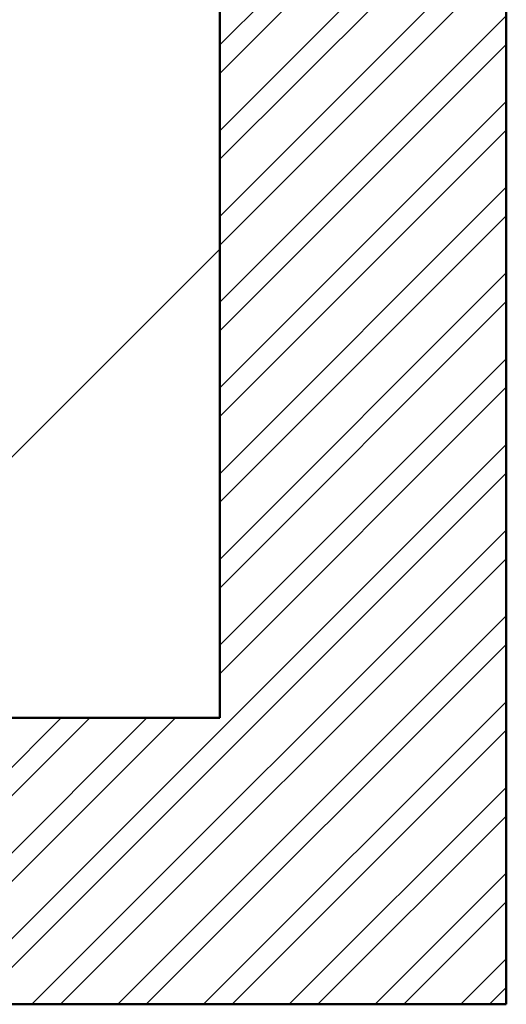
# Model space of a CAD drawing. Units: inches. Extents: x 3590 to 5167, y 65 to 1917.
# Tile 40 of 100: x 5065 to 5080, y 1326 to 1357. Entities that reach past the tile are written whole.
import ezdxf

# ---------------------------------------------------------------- set-up
doc = ezdxf.new("R2010")
doc.units = ezdxf.units.IN
for name, color, linetype, lineweight in [('A-FLOR-PATT', 8, 'Continuous', 13), ('A-WALL', 7, 'Continuous', 50), ('A-WALL-PATT', 251, 'Continuous', 13)]:
    doc.layers.add(name, color=color, linetype=linetype, lineweight=lineweight)

msp = doc.modelspace()

# ---------------------------------------------------------------- hatches: boundary and pattern name
at = {"layer": 'A-FLOR-PATT', "transparency": 33554687}
h = msp.add_hatch(dxfattribs=at)
h.set_pattern_fill('AR-HBONE', color=256, scale=0.2)
h.set_pattern_definition([(45, (-588.972, 0), (0, 28.73682), [60.96, -20.32]), (135, (-574.604, 14.368), (3e-15, 28.73682), [60.96, -20.32])])
h.paths.add_polyline_path([(5071.274, 1796.999), (4933.274, 1796.999), (4933.274, 1753.999), (4962.774, 1753.999, -0.414214), (4928.774, 1719.999), (4933.274, 1718.999), (4933.274, 1334.999), (5071.274, 1334.999)])
h.paths.add_polyline_path([(4951.78, 1521.077), (4951.715, 1521.04), (4951.563, 1520.895)], flags=16)
h.paths.add_polyline_path([(4952.267, 1521.376), (4952.198, 1521.371), (4952.198, 1521.356)], flags=0)
h.paths.add_polyline_path([(4967.051, 1529.728), (4965.231, 1528.694), (4963.411, 1527.714), (4961.756, 1526.851), (4963.589, 1527.449), (4964.036, 1527.478), (4962.975, 1527.249), (4961.76, 1526.852), (4959.792, 1525.834), (4958.005, 1524.895), (4956.24, 1523.93), (4954.504, 1522.919), (4954.129, 1522.682), (4953.361, 1521.997), (4953.366, 1521.998), (4953.605, 1522.064), (4955.106, 1522.761), (4956.921, 1523.434), (4958.678, 1523.915), (4960.358, 1524.2), (4961.945, 1524.286), (4964.171, 1524.108), (4965.958, 1523.309), (4963.863, 1522.976), (4965.187, 1522.499), (4963.366, 1522.497), (4961.545, 1522.487), (4959.764, 1522.461), (4958.304, 1522.419), (4957.974, 1522.388), (4956.307, 1522.232), (4954.718, 1522.071), (4953.251, 1521.899), (4953.525, 1521.623), (4954.331, 1521.379), (4956.243, 1521.23), (4958.039, 1520.93), (4959.684, 1520.483), (4961.16, 1519.896), (4963.107, 1518.8), (4964.393, 1517.325), (4962.973, 1517.726), (4964.558, 1516.661), (4965.407, 1515.708), (4963.507, 1516.322), (4961.68, 1517.005), (4959.935, 1517.745), (4958.282, 1518.528), (4956.732, 1519.343), (4955.295, 1520.175), (4954.672, 1520.572), (4954.513, 1520.627), (4955.658, 1519.318), (4956.703, 1517.982), (4957.644, 1516.647), (4958.485, 1515.334), (4959.55, 1513.524), (4960.438, 1511.769), (4958.841, 1513.62), (4957.452, 1515.325), (4955.819, 1517.459), (4956.665, 1515.448), (4957.111, 1513.923), (4957.447, 1511.714), (4957.076, 1509.793), (4956.538, 1511.11), (4955.992, 1512.569), (4955.444, 1514.125), (4954.898, 1515.735), (4954.357, 1517.356), (4953.824, 1518.943), (4953.305, 1520.452), (4953.065, 1521.116), (4952.971, 1521.146), (4952.949, 1521.086), (4952.73, 1520.199), (4953.37, 1518.024), (4953.757, 1516.373), (4954.051, 1514.765), (4954.264, 1513.221), (4954.471, 1511.131), (4954.497, 1510.402), (4954.409, 1511.76), (4954.264, 1513.221), (4954.051, 1514.765), (4953.757, 1516.373), (4953.37, 1518.024), (4952.877, 1519.698), (4952.716, 1520.141), (4952.533, 1519.059), (4952.374, 1517.789), (4952.219, 1516.312), (4952.046, 1514.6), (4951.833, 1512.626), (4951.557, 1510.363), (4951.203, 1512.168), (4950.852, 1514.339), (4950.985, 1516.376), (4951.66, 1518.286), (4952.593, 1520.481), (4952.357, 1521.13), (4951.855, 1520.328), (4950.839, 1518.908), (4949.777, 1517.587), (4948.916, 1516.617), (4948.111, 1515.256), (4947.089, 1513.554), (4945.889, 1511.615), (4946.326, 1513.402), (4946.562, 1514.249), (4945.528, 1513.327), (4944.581, 1512.531), (4946.018, 1514.508), (4947.204, 1516.048), (4947.893, 1517.313), (4949.307, 1518.764), (4950.414, 1519.767), (4950.451, 1519.806), (4952.267, 1521.376), (4951.645, 1521.493), (4950.404, 1521.18), (4948.044, 1520.359), (4946.119, 1519.452), (4944.572, 1518.475), (4943.35, 1517.443), (4941.997, 1515.92), (4941.661, 1515.275), (4942.813, 1516.99), (4944.572, 1518.475), (4946.119, 1519.452), (4948.044, 1520.359), (4950.404, 1521.18), (4951.645, 1521.493), (4949.647, 1521.868), (4948.6, 1521.756), (4947.126, 1521.57), (4945.42, 1521.348), (4943.45, 1521.105), (4941.183, 1520.856), (4942.86, 1521.613), (4943.873, 1522.03), (4942.952, 1521.909), (4941.41, 1521.485), (4939.543, 1520.67), (4938.968, 1520.226), (4940.733, 1521.299), (4942.952, 1521.909), (4943.702, 1522.008), (4945.894, 1522.7), (4947.565, 1522.714), (4948.921, 1522.566), (4951.131, 1522.183), (4950.971, 1522.297), (4948.129, 1523.006), (4946.035, 1523.707), (4944.232, 1524.521), (4942.707, 1525.461), (4941.444, 1526.537), (4940.43, 1527.761), (4939.649, 1529.143), (4941.421, 1528.122), (4943.147, 1527.132), (4944.841, 1526.175), (4946.514, 1525.25), (4948.179, 1524.359), (4948.365, 1524.263), (4946.475, 1526.045), (4945.181, 1527.54), (4944.19, 1529.033), (4943.496, 1530.54), (4943.278, 1531.36), (4942.498, 1531.919), (4943.114, 1531.762), (4942.959, 1533.659), (4944.14, 1531.989), (4944.612, 1531.323), (4946.202, 1530.463), (4947.486, 1529.509), (4948.79, 1528.226), (4950.368, 1526.237), (4949.485, 1528.155), (4948.851, 1530.123), (4948.491, 1532.041), (4948.381, 1533.918), (4948.501, 1535.76), (4948.827, 1537.573), (4949.418, 1535.565), (4949.957, 1533.569), (4950.464, 1531.586), (4950.961, 1529.617), (4951.391, 1527.954), (4951.724, 1530.687), (4952.201, 1532.58), (4952.889, 1534.33), (4953.77, 1535.951), (4954.827, 1537.46), (4954.521, 1535.39), (4954.273, 1533.937), (4955.58, 1535.663), (4956.748, 1536.739), (4956.159, 1534.78), (4955.589, 1532.873), (4955.043, 1531.006), (4954.525, 1529.166), (4954.038, 1527.341), (4953.638, 1525.733), (4953.611, 1525.586), (4953.398, 1524.166), (4953.382, 1524.009), (4954.07, 1525.476), (4954.912, 1527.022), (4956.136, 1528.894), (4957.847, 1530.577), (4959.376, 1531.54), (4958.256, 1530.104), (4957.143, 1528.663), (4956.066, 1527.243), (4955.056, 1525.871), (4954.141, 1524.571), (4953.352, 1523.372), (4953.311, 1523.303), (4953.273, 1522.925), (4953.261, 1522.382), (4954.103, 1523.373), (4954.63, 1524.284), (4955.961, 1526.358), (4957.23, 1528.13), (4958.421, 1529.609), (4960.037, 1531.368), (4961.374, 1532.375), (4962.101, 1532.77), (4961.07, 1531.061), (4959.987, 1529.438), (4958.869, 1527.908), (4958.15, 1527.007), (4959.803, 1528.003), (4961.589, 1528.793), (4963.391, 1529.328), (4965.211, 1529.632)], flags=16)
h.paths.add_polyline_path([(4962.944, 1523.182), (4961.107, 1523.422), (4960.392, 1523.362), (4962.35, 1523.331)], flags=0)
h.paths.add_polyline_path([(5049.541, 1584.551), (5049.476, 1584.515), (5049.325, 1584.37)], flags=16)
h.paths.add_polyline_path([(5050.028, 1584.851), (5049.959, 1584.845), (5049.959, 1584.83)], flags=0)
h.paths.add_polyline_path([(5042.333, 1581.949), (5043.88, 1582.926), (5045.806, 1583.833), (5048.165, 1584.654), (5049.406, 1584.967), (5047.408, 1585.342), (5046.361, 1585.231), (5044.888, 1585.044), (5043.181, 1584.822), (5041.211, 1584.579), (5038.944, 1584.33), (5040.622, 1585.087), (5041.634, 1585.504), (5040.713, 1585.383), (5039.171, 1584.959), (5037.304, 1584.144), (5036.729, 1583.7), (5038.494, 1584.773), (5040.713, 1585.383), (5041.463, 1585.482), (5043.655, 1586.174), (5045.326, 1586.188), (5046.682, 1586.04), (5048.893, 1585.657), (5048.732, 1585.771), (5045.891, 1586.48), (5043.796, 1587.181), (5041.994, 1587.996), (5040.468, 1588.935), (5039.205, 1590.011), (5038.191, 1591.235), (5037.41, 1592.617), (5039.182, 1591.596), (5040.909, 1590.607), (5042.602, 1589.649), (5044.275, 1588.724), (5045.94, 1587.833), (5046.126, 1587.738), (5044.237, 1589.519), (5042.942, 1591.015), (5041.952, 1592.508), (5041.257, 1594.014), (5041.039, 1594.834), (5040.26, 1595.393), (5040.875, 1595.237), (5040.721, 1597.133), (5041.901, 1595.463), (5042.373, 1594.798), (5043.963, 1593.938), (5045.247, 1592.983), (5046.552, 1591.701), (5048.129, 1589.712), (5047.247, 1591.63), (5046.613, 1593.597), (5046.252, 1595.515), (5046.142, 1597.392), (5046.262, 1599.234), (5046.588, 1601.047), (5047.179, 1599.039), (5047.718, 1597.043), (5048.225, 1595.06), (5048.722, 1593.091), (5049.152, 1591.429), (5049.485, 1594.161), (5049.962, 1596.054), (5050.65, 1597.804), (5051.532, 1599.425), (5052.589, 1600.934), (5052.283, 1598.864), (5052.034, 1597.411), (5053.341, 1599.137), (5054.509, 1600.213), (5053.92, 1598.254), (5053.35, 1596.348), (5052.805, 1594.48), (5052.286, 1592.64), (5051.799, 1590.815), (5051.4, 1589.207), (5051.373, 1589.06), (5051.159, 1587.64), (5051.143, 1587.483), (5051.831, 1588.95), (5052.673, 1590.496), (5053.898, 1592.368), (5055.608, 1594.051), (5057.137, 1595.014), (5056.017, 1593.578), (5054.904, 1592.137), (5053.828, 1590.717), (5052.817, 1589.345), (5051.902, 1588.046), (5051.113, 1586.846), (5051.072, 1586.777), (5051.034, 1586.399), (5051.022, 1585.856), (5051.864, 1586.847), (5052.391, 1587.758), (5053.723, 1589.832), (5054.991, 1591.604), (5056.182, 1593.083), (5057.798, 1594.842), (5059.135, 1595.849), (5059.863, 1596.244), (5058.831, 1594.535), (5057.749, 1592.912), (5056.63, 1591.382), (5055.912, 1590.482), (5057.564, 1591.477), (5059.35, 1592.267), (5061.152, 1592.802), (5062.972, 1593.106), (5064.812, 1593.203), (5062.992, 1592.169), (5061.172, 1591.188), (5059.518, 1590.325), (5061.35, 1590.924), (5061.797, 1590.952), (5060.737, 1590.723), (5059.521, 1590.326), (5057.553, 1589.308), (5055.766, 1588.369), (5054.002, 1587.404), (5052.265, 1586.393), (5051.891, 1586.156), (5051.122, 1585.471), (5051.127, 1585.472), (5051.366, 1585.538), (5052.867, 1586.235), (5054.682, 1586.908), (5056.439, 1587.389), (5058.12, 1587.675), (5059.706, 1587.76), (5061.933, 1587.583), (5063.719, 1586.783), (5061.624, 1586.45), (5062.949, 1585.973), (5061.127, 1585.971), (5059.307, 1585.961), (5057.525, 1585.935), (5056.065, 1585.893), (5055.735, 1585.862), (5054.068, 1585.707), (5052.479, 1585.546), (5051.012, 1585.373), (5051.286, 1585.097), (5052.092, 1584.853), (5054.004, 1584.704), (5055.8, 1584.404), (5057.446, 1583.958), (5058.921, 1583.37), (5060.868, 1582.274), (5062.154, 1580.799), (5060.734, 1581.2), (5062.32, 1580.135), (5063.168, 1579.182), (5061.269, 1579.796), (5059.441, 1580.479), (5057.696, 1581.219), (5056.043, 1582.003), (5054.493, 1582.817), (5053.057, 1583.649), (5052.433, 1584.047), (5052.274, 1584.101), (5053.42, 1582.793), (5054.464, 1581.457), (5055.405, 1580.121), (5056.247, 1578.809), (5057.311, 1576.998), (5058.199, 1575.244), (5056.602, 1577.094), (5055.213, 1578.799), (5053.58, 1580.933), (5054.427, 1578.922), (5054.872, 1577.397), (5055.208, 1575.189), (5054.838, 1573.267), (5054.299, 1574.584), (5053.754, 1576.043), (5053.206, 1577.599), (5052.659, 1579.209), (5052.118, 1580.83), (5051.585, 1582.417), (5051.066, 1583.927), (5050.826, 1584.59), (5050.733, 1584.62), (5050.711, 1584.561), (5050.491, 1583.673), (5051.131, 1581.498), (5051.518, 1579.847), (5051.813, 1578.24), (5052.026, 1576.695), (5052.233, 1574.605), (5052.258, 1573.876), (5052.17, 1575.234), (5052.026, 1576.695), (5051.813, 1578.24), (5051.518, 1579.847), (5051.131, 1581.498), (5050.638, 1583.172), (5050.477, 1583.615), (5050.294, 1582.533), (5050.136, 1581.263), (5049.981, 1579.786), (5049.807, 1578.074), (5049.594, 1576.1), (5049.318, 1573.837), (5048.965, 1575.642), (5048.613, 1577.813), (5048.747, 1579.85), (5049.421, 1581.76), (5050.354, 1583.955), (5050.118, 1584.604), (5049.616, 1583.802), (5048.6, 1582.382), (5047.538, 1581.061), (5046.677, 1580.091), (5045.872, 1578.73), (5044.85, 1577.028), (5043.651, 1575.089), (5044.087, 1576.877), (5044.324, 1577.723), (5043.289, 1576.801), (5042.342, 1576.005), (5043.779, 1577.982), (5044.966, 1579.522), (5045.655, 1580.787), (5047.068, 1582.239), (5048.175, 1583.241), (5048.213, 1583.28), (5050.028, 1584.851), (5049.406, 1584.967), (5048.165, 1584.654), (5045.806, 1583.833), (5043.88, 1582.926), (5042.333, 1581.949), (5041.111, 1580.917), (5039.758, 1579.394), (5039.423, 1578.749), (5040.575, 1580.464)], flags=16)
h.paths.add_polyline_path([(4954.799, 1533.12), (4954.262, 1532.079), (4953.831, 1530.935), (4953.505, 1529.636), (4953.283, 1528.133), (4953.167, 1526.376), (4953.156, 1524.315), (4953.277, 1521.236), (4952.802, 1521.842), (4951.557, 1521.998), (4950.976, 1521.961), (4952.661, 1521.941), (4952.802, 1521.842), (4953.152, 1523.593), (4953.167, 1526.376), (4953.283, 1528.133), (4953.609, 1530.346), (4954.456, 1532.592)], flags=0)
h.paths.add_polyline_path([(5050.563, 1585.316), (5049.318, 1585.472), (5048.737, 1585.435), (5050.422, 1585.415), (5050.563, 1585.316), (5050.914, 1587.067), (5050.928, 1589.851), (5051.045, 1591.607), (5051.371, 1593.82), (5052.217, 1596.066), (5052.56, 1596.594), (5052.024, 1595.554), (5051.592, 1594.409), (5051.266, 1593.11), (5051.045, 1591.607), (5050.928, 1589.851), (5050.918, 1587.789), (5051.038, 1584.71)], flags=0)
h.paths.add_polyline_path([(5058.153, 1586.836), (5060.111, 1586.805), (5060.705, 1586.656), (5058.868, 1586.896)], flags=0)
h.paths.add_polyline_path([(5049.541, 1430.936), (5049.476, 1430.9), (5049.325, 1430.755)], flags=16)
h.paths.add_polyline_path([(5050.028, 1431.236), (5049.959, 1431.231), (5049.959, 1431.215)], flags=0)
h.paths.add_polyline_path([(5046.588, 1447.432), (5047.179, 1445.425), (5047.718, 1443.429), (5048.225, 1441.446), (5048.722, 1439.476), (5049.152, 1437.814), (5049.485, 1440.546), (5049.962, 1442.439), (5050.65, 1444.189), (5051.532, 1445.811), (5052.589, 1447.319), (5052.283, 1445.249), (5052.034, 1443.796), (5053.341, 1445.522), (5054.509, 1446.598), (5053.92, 1444.64), (5053.35, 1442.733), (5052.805, 1440.865), (5052.286, 1439.025), (5051.799, 1437.201), (5051.4, 1435.592), (5051.373, 1435.445), (5051.159, 1434.025), (5051.143, 1433.868), (5051.831, 1435.335), (5052.673, 1436.881), (5053.898, 1438.753), (5055.608, 1440.436), (5057.137, 1441.4), (5056.017, 1439.963), (5054.904, 1438.522), (5053.828, 1437.102), (5052.817, 1435.73), (5051.902, 1434.431), (5051.113, 1433.231), (5051.072, 1433.162), (5051.034, 1432.784), (5051.022, 1432.242), (5051.864, 1433.232), (5052.391, 1434.143), (5053.723, 1436.217), (5054.991, 1437.989), (5056.182, 1439.468), (5057.798, 1441.227), (5059.135, 1442.235), (5059.863, 1442.629), (5058.831, 1440.921), (5057.749, 1439.298), (5056.63, 1437.767), (5055.912, 1436.867), (5057.564, 1437.863), (5059.35, 1438.652), (5061.152, 1439.187), (5062.972, 1439.491), (5064.812, 1439.588), (5062.992, 1438.554), (5061.172, 1437.573), (5059.518, 1436.71), (5061.35, 1437.309), (5061.797, 1437.337), (5060.737, 1437.108), (5059.521, 1436.711), (5057.553, 1435.693), (5055.766, 1434.754), (5054.002, 1433.789), (5052.265, 1432.778), (5051.891, 1432.541), (5051.122, 1431.856), (5051.127, 1431.857), (5051.366, 1431.923), (5052.867, 1432.62), (5054.682, 1433.293), (5056.439, 1433.775), (5058.12, 1434.06), (5059.706, 1434.145), (5061.933, 1433.968), (5063.719, 1433.168), (5061.624, 1432.835), (5062.949, 1432.358), (5061.127, 1432.357), (5059.307, 1432.346), (5057.525, 1432.32), (5056.065, 1432.278), (5055.735, 1432.248), (5054.068, 1432.092), (5052.479, 1431.931), (5051.012, 1431.759), (5051.286, 1431.482), (5052.092, 1431.238), (5054.004, 1431.089), (5055.8, 1430.789), (5057.446, 1430.343), (5058.921, 1429.755), (5060.868, 1428.66), (5062.154, 1427.185), (5060.734, 1427.585), (5062.32, 1426.52), (5063.168, 1425.567), (5061.269, 1426.181), (5059.441, 1426.865), (5057.696, 1427.604), (5056.043, 1428.388), (5054.493, 1429.202), (5053.057, 1430.034), (5052.433, 1430.432), (5052.274, 1430.487), (5053.42, 1429.178), (5054.464, 1427.842), (5055.405, 1426.506), (5056.247, 1425.194), (5057.311, 1423.383), (5058.199, 1421.629), (5056.602, 1423.479), (5055.213, 1425.184), (5053.58, 1427.318), (5054.427, 1425.307), (5054.872, 1423.782), (5055.208, 1421.574), (5054.838, 1419.652), (5054.299, 1420.97), (5053.754, 1422.428), (5053.206, 1423.984), (5052.659, 1425.595), (5052.118, 1427.215), (5051.585, 1428.802), (5051.066, 1430.312), (5050.826, 1430.975), (5050.733, 1431.005), (5050.711, 1430.946), (5050.491, 1430.058), (5051.131, 1427.883), (5051.518, 1426.232), (5051.813, 1424.625), (5052.026, 1423.081), (5052.233, 1420.991), (5052.258, 1420.261), (5052.17, 1421.619), (5052.026, 1423.081), (5051.813, 1424.625), (5051.518, 1426.232), (5051.131, 1427.883), (5050.638, 1429.558), (5050.477, 1430.001), (5050.294, 1428.918), (5050.136, 1427.648), (5049.981, 1426.171), (5049.807, 1424.459), (5049.594, 1422.485), (5049.318, 1420.222), (5048.965, 1422.028), (5048.613, 1424.199), (5048.747, 1426.235), (5049.421, 1428.146), (5050.354, 1430.34), (5050.118, 1430.989), (5049.616, 1430.187), (5048.6, 1428.768), (5047.538, 1427.446), (5046.677, 1426.477), (5045.872, 1425.116), (5044.85, 1423.413), (5043.651, 1421.474), (5044.087, 1423.262), (5044.324, 1424.109), (5043.289, 1423.186), (5042.342, 1422.391), (5043.779, 1424.368), (5044.966, 1425.907), (5045.655, 1427.173), (5047.068, 1428.624), (5048.175, 1429.627), (5048.213, 1429.666), (5050.028, 1431.236), (5049.406, 1431.353), (5048.165, 1431.039), (5045.806, 1430.218), (5043.88, 1429.311), (5042.333, 1428.334), (5041.111, 1427.302), (5039.758, 1425.779), (5039.423, 1425.134), (5040.575, 1426.849), (5042.333, 1428.334), (5043.88, 1429.311), (5045.806, 1430.218), (5048.165, 1431.039), (5049.406, 1431.353), (5047.408, 1431.727), (5046.361, 1431.616), (5044.888, 1431.429), (5043.181, 1431.207), (5041.211, 1430.964), (5038.944, 1430.715), (5040.622, 1431.472), (5041.634, 1431.89), (5040.713, 1431.769), (5039.171, 1431.345), (5037.304, 1430.53), (5036.729, 1430.085), (5038.494, 1431.158), (5040.713, 1431.769), (5041.463, 1431.867), (5043.655, 1432.559), (5045.326, 1432.573), (5046.682, 1432.425), (5048.893, 1432.042), (5048.732, 1432.156), (5045.891, 1432.865), (5043.796, 1433.566), (5041.994, 1434.381), (5040.468, 1435.321), (5039.205, 1436.396), (5038.191, 1437.62), (5037.41, 1439.002), (5039.182, 1437.982), (5040.909, 1436.992), (5042.602, 1436.034), (5044.275, 1435.109), (5045.94, 1434.218), (5046.126, 1434.123), (5044.237, 1435.904), (5042.942, 1437.4), (5041.952, 1438.893), (5041.257, 1440.399), (5041.039, 1441.219), (5040.26, 1441.778), (5040.875, 1441.622), (5040.721, 1443.518), (5041.901, 1441.848), (5042.373, 1441.183), (5043.963, 1440.323), (5045.247, 1439.369), (5046.552, 1438.086), (5048.129, 1436.097), (5047.247, 1438.015), (5046.613, 1439.982), (5046.252, 1441.901), (5046.142, 1443.778), (5046.262, 1445.619)], flags=16)
h.paths.add_polyline_path([(5052.382, 1444.255), (5051.623, 1442.78), (5052.024, 1441.939), (5052.56, 1442.98)], flags=0)
h.paths.add_polyline_path([(5050.563, 1431.701), (5049.318, 1431.857), (5048.737, 1431.821), (5050.422, 1431.8)], flags=0)
h.paths.add_polyline_path([(5058.153, 1433.221), (5060.111, 1433.19), (5060.705, 1433.041), (5058.868, 1433.281)], flags=0)
h.paths.add_polyline_path([(5049.541, 1352.285), (5049.476, 1352.249), (5049.325, 1352.104)], flags=16)
h.paths.add_polyline_path([(5050.028, 1352.585), (5049.959, 1352.58), (5049.959, 1352.564)], flags=0)
h.paths.add_polyline_path([(5046.588, 1368.781), (5047.179, 1366.774), (5047.718, 1364.778), (5048.225, 1362.795), (5048.722, 1360.825), (5049.152, 1359.163), (5049.485, 1361.896), (5049.962, 1363.789), (5050.65, 1365.538), (5051.532, 1367.16), (5052.589, 1368.669), (5052.283, 1366.598), (5052.034, 1365.145), (5053.341, 1366.871), (5054.509, 1367.947), (5053.92, 1365.989), (5053.35, 1364.082), (5052.805, 1362.214), (5052.286, 1360.374), (5051.799, 1358.55), (5051.4, 1356.942), (5051.373, 1356.794), (5051.159, 1355.374), (5051.143, 1355.218), (5051.831, 1356.684), (5052.673, 1358.23), (5053.898, 1360.102), (5055.608, 1361.786), (5057.137, 1362.749), (5056.017, 1361.313), (5054.904, 1359.872), (5053.828, 1358.452), (5052.817, 1357.079), (5051.902, 1355.78), (5051.113, 1354.581), (5051.072, 1354.512), (5051.034, 1354.133), (5051.022, 1353.591), (5051.864, 1354.581), (5052.391, 1355.492), (5053.723, 1357.566), (5054.991, 1359.338), (5056.182, 1360.817), (5057.798, 1362.577), (5059.135, 1363.584), (5059.863, 1363.979), (5058.831, 1362.27), (5057.749, 1360.647), (5056.63, 1359.117), (5055.912, 1358.216), (5057.564, 1359.212), (5059.35, 1360.001), (5061.152, 1360.536), (5062.972, 1360.841), (5064.812, 1360.937), (5062.992, 1359.903), (5061.172, 1358.923), (5059.518, 1358.059), (5061.35, 1358.658), (5061.797, 1358.687), (5060.737, 1358.458), (5059.521, 1358.061), (5057.553, 1357.043), (5055.766, 1356.103), (5054.002, 1355.138), (5052.265, 1354.127), (5051.891, 1353.89), (5051.122, 1353.206), (5051.127, 1353.206), (5051.366, 1353.272), (5052.867, 1353.969), (5054.682, 1354.643), (5056.439, 1355.124), (5058.12, 1355.409), (5059.706, 1355.495), (5061.933, 1355.317), (5063.719, 1354.518), (5061.624, 1354.184), (5062.949, 1353.708), (5061.127, 1353.706), (5059.307, 1353.695), (5057.525, 1353.669), (5056.065, 1353.627), (5055.735, 1353.597), (5054.068, 1353.441), (5052.479, 1353.28), (5051.012, 1353.108), (5051.286, 1352.831), (5052.092, 1352.587), (5054.004, 1352.439), (5055.8, 1352.138), (5057.446, 1351.692), (5058.921, 1351.104), (5060.868, 1350.009), (5062.154, 1348.534), (5060.734, 1348.935), (5062.32, 1347.869), (5063.168, 1346.916), (5061.269, 1347.53), (5059.441, 1348.214), (5057.696, 1348.954), (5056.043, 1349.737), (5054.493, 1350.551), (5053.057, 1351.383), (5052.433, 1351.781), (5052.274, 1351.836), (5053.42, 1350.527), (5054.464, 1349.191), (5055.405, 1347.855), (5056.247, 1346.543), (5057.311, 1344.733), (5058.199, 1342.978), (5056.602, 1344.828), (5055.213, 1346.534), (5053.58, 1348.667), (5054.427, 1346.656), (5054.872, 1345.132), (5055.208, 1342.923), (5054.838, 1341.002), (5054.299, 1342.319), (5053.754, 1343.778), (5053.206, 1345.334), (5052.659, 1346.944), (5052.118, 1348.564), (5051.585, 1350.151), (5051.066, 1351.661), (5050.826, 1352.324), (5050.733, 1352.355), (5050.711, 1352.295), (5050.491, 1351.408), (5051.131, 1349.232), (5051.518, 1347.581), (5051.813, 1345.974), (5052.026, 1344.43), (5052.233, 1342.34), (5052.258, 1341.61), (5052.17, 1342.969), (5052.026, 1344.43), (5051.813, 1345.974), (5051.518, 1347.581), (5051.131, 1349.232), (5050.638, 1350.907), (5050.477, 1351.35), (5050.294, 1350.267), (5050.136, 1348.997), (5049.981, 1347.52), (5049.807, 1345.809), (5049.594, 1343.835), (5049.318, 1341.571), (5048.965, 1343.377), (5048.613, 1345.548), (5048.747, 1347.585), (5049.421, 1349.495), (5050.354, 1351.689), (5050.118, 1352.339), (5049.616, 1351.536), (5048.6, 1350.117), (5047.538, 1348.795), (5046.677, 1347.826), (5045.872, 1346.465), (5044.85, 1344.763), (5043.651, 1342.824), (5044.087, 1344.611), (5044.324, 1345.458), (5043.289, 1344.535), (5042.342, 1343.74), (5043.779, 1345.717), (5044.966, 1347.256), (5045.655, 1348.522), (5047.068, 1349.973), (5048.175, 1350.976), (5048.213, 1351.015), (5050.028, 1352.585), (5049.406, 1352.702), (5048.165, 1352.388), (5045.806, 1351.567), (5043.88, 1350.661), (5042.333, 1349.683), (5041.111, 1348.651), (5039.758, 1347.128), (5039.423, 1346.483), (5040.575, 1348.198), (5042.333, 1349.683), (5043.88, 1350.661), (5045.806, 1351.567), (5048.165, 1352.388), (5049.406, 1352.702), (5047.408, 1353.076), (5046.361, 1352.965), (5044.888, 1352.779), (5043.181, 1352.556), (5041.211, 1352.313), (5038.944, 1352.065), (5040.622, 1352.821), (5041.634, 1353.239), (5040.713, 1353.118), (5039.171, 1352.694), (5037.304, 1351.879), (5036.729, 1351.434), (5038.494, 1352.508), (5040.713, 1353.118), (5041.463, 1353.216), (5043.655, 1353.909), (5045.326, 1353.923), (5046.682, 1353.774), (5048.893, 1353.391), (5048.732, 1353.506), (5045.891, 1354.214), (5043.796, 1354.915), (5041.994, 1355.73), (5040.468, 1356.67), (5039.205, 1357.746), (5038.191, 1358.969), (5037.41, 1360.352), (5039.182, 1359.331), (5040.909, 1358.341), (5042.602, 1357.383), (5044.275, 1356.458), (5045.94, 1355.567), (5046.126, 1355.472), (5044.237, 1357.253), (5042.942, 1358.749), (5041.952, 1360.242), (5041.257, 1361.748), (5041.039, 1362.568), (5040.26, 1363.128), (5040.875, 1362.971), (5040.721, 1364.867), (5041.901, 1363.197), (5042.373, 1362.532), (5043.963, 1361.672), (5045.247, 1360.718), (5046.552, 1359.435), (5048.129, 1357.446), (5047.247, 1359.364), (5046.613, 1361.331), (5046.252, 1363.25), (5046.142, 1365.127), (5046.262, 1366.969)], flags=16)
h.paths.add_polyline_path([(5052.382, 1365.604), (5051.623, 1364.129), (5052.024, 1363.288), (5052.56, 1364.329)], flags=0)
h.paths.add_polyline_path([(4951.78, 1698.041), (4951.715, 1698.005), (4951.563, 1697.859)], flags=16)
h.paths.add_polyline_path([(4952.267, 1698.341), (4952.198, 1698.335), (4952.198, 1698.32)], flags=0)
h.paths.add_polyline_path([(4957.076, 1686.757), (4956.538, 1688.074), (4955.992, 1689.533), (4955.444, 1691.089), (4954.898, 1692.699), (4954.357, 1694.32), (4953.824, 1695.907), (4953.305, 1697.417), (4953.065, 1698.08), (4952.971, 1698.11), (4952.949, 1698.051), (4952.73, 1697.163), (4953.37, 1694.988), (4953.757, 1693.337), (4954.051, 1691.729), (4954.264, 1690.185), (4954.471, 1688.095), (4954.497, 1687.366), (4954.409, 1688.724), (4954.264, 1690.185), (4954.051, 1691.729), (4953.757, 1693.337), (4953.37, 1694.988), (4952.877, 1696.662), (4952.716, 1697.105), (4952.533, 1696.023), (4952.374, 1694.753), (4952.219, 1693.276), (4952.046, 1691.564), (4951.833, 1689.59), (4951.557, 1687.327), (4951.203, 1689.132), (4950.852, 1691.303), (4950.985, 1693.34), (4951.66, 1695.25), (4952.593, 1697.445), (4952.357, 1698.094), (4951.855, 1697.292), (4950.839, 1695.872), (4949.777, 1694.551), (4948.916, 1693.581), (4948.111, 1692.22), (4947.089, 1690.518), (4945.889, 1688.579), (4946.326, 1690.366), (4946.562, 1691.213), (4945.528, 1690.291), (4944.581, 1689.495), (4946.018, 1691.472), (4947.204, 1693.012), (4947.893, 1694.277), (4949.307, 1695.729), (4950.414, 1696.731), (4950.451, 1696.77), (4952.267, 1698.341), (4951.645, 1698.457), (4950.404, 1698.144), (4948.044, 1697.323), (4946.119, 1696.416), (4944.572, 1695.439), (4943.35, 1694.407), (4941.997, 1692.884), (4941.661, 1692.239), (4942.813, 1693.954), (4944.572, 1695.439), (4946.119, 1696.416), (4948.044, 1697.323), (4950.404, 1698.144), (4951.645, 1698.457), (4949.647, 1698.832), (4948.6, 1698.72), (4947.126, 1698.534), (4945.42, 1698.312), (4943.45, 1698.069), (4941.183, 1697.82), (4942.86, 1698.577), (4943.873, 1698.994), (4942.952, 1698.873), (4941.41, 1698.449), (4939.543, 1697.634), (4938.968, 1697.19), (4940.733, 1698.263), (4942.952, 1698.873), (4943.702, 1698.972), (4945.894, 1699.664), (4947.565, 1699.678), (4948.921, 1699.53), (4951.131, 1699.147), (4950.971, 1699.261), (4948.129, 1699.97), (4946.035, 1700.671), (4944.232, 1701.486), (4942.707, 1702.425), (4941.444, 1703.501), (4940.43, 1704.725), (4939.649, 1706.107), (4941.421, 1705.086), (4943.147, 1704.097), (4944.841, 1703.139), (4946.514, 1702.214), (4948.179, 1701.323), (4948.365, 1701.227), (4946.475, 1703.009), (4945.181, 1704.505), (4944.19, 1705.997), (4943.496, 1707.504), (4943.278, 1708.324), (4942.498, 1708.883), (4943.114, 1708.727), (4942.959, 1710.623), (4944.14, 1708.953), (4944.612, 1708.287), (4946.202, 1707.428), (4947.486, 1706.473), (4948.79, 1705.191), (4950.368, 1703.202), (4949.485, 1705.12), (4948.851, 1707.087), (4948.491, 1709.005), (4948.381, 1710.882), (4948.501, 1712.724), (4948.827, 1714.537), (4949.418, 1712.529), (4949.957, 1710.533), (4950.464, 1708.55), (4950.961, 1706.581), (4951.391, 1704.919), (4951.724, 1707.651), (4952.201, 1709.544), (4952.889, 1711.294), (4953.77, 1712.915), (4954.827, 1714.424), (4954.521, 1712.354), (4954.273, 1710.901), (4955.58, 1712.627), (4956.748, 1713.703), (4956.159, 1711.744), (4955.589, 1709.837), (4955.043, 1707.97), (4954.525, 1706.13), (4954.038, 1704.305), (4953.638, 1702.697), (4953.611, 1702.55), (4953.398, 1701.13), (4953.382, 1700.973), (4954.07, 1702.44), (4954.912, 1703.986), (4956.136, 1705.858), (4957.847, 1707.541), (4959.376, 1708.504), (4958.256, 1707.068), (4957.143, 1705.627), (4956.066, 1704.207), (4955.056, 1702.835), (4954.141, 1701.536), (4953.352, 1700.336), (4953.311, 1700.267), (4953.273, 1699.889), (4953.261, 1699.346), (4954.103, 1700.337), (4954.63, 1701.248), (4955.961, 1703.322), (4957.23, 1705.094), (4958.421, 1706.573), (4960.037, 1708.332), (4961.374, 1709.339), (4962.101, 1709.734), (4961.07, 1708.025), (4959.987, 1706.402), (4958.869, 1704.872), (4958.15, 1703.972), (4959.803, 1704.967), (4961.589, 1705.757), (4963.391, 1706.292), (4965.211, 1706.596), (4967.051, 1706.692), (4965.231, 1705.659), (4963.411, 1704.678), (4961.756, 1703.815), (4963.589, 1704.413), (4964.036, 1704.442), (4962.975, 1704.213), (4961.76, 1703.816), (4959.792, 1702.798), (4958.005, 1701.859), (4956.24, 1700.894), (4954.504, 1699.883), (4954.129, 1699.646), (4953.361, 1698.961), (4953.366, 1698.962), (4953.605, 1699.028), (4955.106, 1699.725), (4956.921, 1700.398), (4958.678, 1700.879), (4960.358, 1701.164), (4961.945, 1701.25), (4964.171, 1701.073), (4965.958, 1700.273), (4963.863, 1699.94), (4965.187, 1699.463), (4963.366, 1699.461), (4961.545, 1699.451), (4959.764, 1699.425), (4958.304, 1699.383), (4957.974, 1699.352), (4956.307, 1699.197), (4954.718, 1699.036), (4953.251, 1698.863), (4953.525, 1698.587), (4954.331, 1698.343), (4956.243, 1698.194), (4958.039, 1697.894), (4959.684, 1697.447), (4961.16, 1696.86), (4963.107, 1695.764), (4964.393, 1694.289), (4962.973, 1694.69), (4964.558, 1693.625), (4965.407, 1692.672), (4963.507, 1693.286), (4961.68, 1693.969), (4959.935, 1694.709), (4958.282, 1695.492), (4956.732, 1696.307), (4955.295, 1697.139), (4954.672, 1697.536), (4954.513, 1697.591), (4955.658, 1696.282), (4956.703, 1694.946), (4957.644, 1693.611), (4958.485, 1692.298), (4959.55, 1690.488), (4960.438, 1688.733), (4958.841, 1690.584), (4957.452, 1692.289), (4955.819, 1694.423), (4956.665, 1692.412), (4957.111, 1690.887), (4957.447, 1688.678)], flags=16)
h.paths.add_polyline_path([(5050.563, 1353.05), (5049.318, 1353.207), (5048.737, 1353.17), (5050.422, 1353.15)], flags=0)
h.paths.add_polyline_path([(4951.78, 1351.486), (4951.715, 1351.45), (4951.563, 1351.305)], flags=16)
h.paths.add_polyline_path([(4952.267, 1351.786), (4952.198, 1351.78), (4952.198, 1351.765)], flags=0)
h.paths.add_polyline_path([(4954.827, 1367.869), (4954.521, 1365.799), (4954.273, 1364.346), (4955.58, 1366.072), (4956.748, 1367.148), (4956.159, 1365.19), (4955.589, 1363.283), (4955.043, 1361.415), (4954.525, 1359.575), (4954.038, 1357.751), (4953.638, 1356.142), (4953.611, 1355.995), (4953.398, 1354.575), (4953.382, 1354.418), (4954.07, 1355.885), (4954.912, 1357.431), (4956.136, 1359.303), (4957.847, 1360.986), (4959.376, 1361.95), (4958.256, 1360.513), (4957.143, 1359.072), (4956.066, 1357.652), (4955.056, 1356.28), (4954.141, 1354.981), (4953.352, 1353.781), (4953.311, 1353.712), (4953.273, 1353.334), (4953.261, 1352.792), (4954.103, 1353.782), (4954.63, 1354.693), (4955.961, 1356.767), (4957.23, 1358.539), (4958.421, 1360.018), (4960.037, 1361.777), (4961.374, 1362.785), (4962.101, 1363.179), (4961.07, 1361.471), (4959.987, 1359.848), (4958.869, 1358.317), (4958.15, 1357.417), (4959.803, 1358.413), (4961.589, 1359.202), (4963.391, 1359.737), (4965.211, 1360.041), (4967.051, 1360.138), (4965.231, 1359.104), (4963.411, 1358.123), (4961.756, 1357.26), (4963.589, 1357.859), (4964.036, 1357.887), (4962.975, 1357.658), (4961.76, 1357.261), (4959.792, 1356.243), (4958.005, 1355.304), (4956.24, 1354.339), (4954.504, 1353.328), (4954.129, 1353.091), (4953.361, 1352.406), (4953.366, 1352.407), (4953.605, 1352.473), (4955.106, 1353.17), (4956.921, 1353.843), (4958.678, 1354.325), (4960.358, 1354.61), (4961.945, 1354.695), (4964.171, 1354.518), (4965.958, 1353.718), (4963.863, 1353.385), (4965.187, 1352.908), (4963.366, 1352.907), (4961.545, 1352.896), (4959.764, 1352.87), (4958.304, 1352.828), (4957.974, 1352.798), (4956.307, 1352.642), (4954.718, 1352.481), (4953.251, 1352.309), (4953.525, 1352.032), (4954.331, 1351.788), (4956.243, 1351.639), (4958.039, 1351.339), (4959.684, 1350.893), (4961.16, 1350.305), (4963.107, 1349.21), (4964.393, 1347.735), (4962.973, 1348.135), (4964.558, 1347.07), (4965.407, 1346.117), (4963.507, 1346.731), (4961.68, 1347.414), (4959.935, 1348.154), (4958.282, 1348.938), (4956.732, 1349.752), (4955.295, 1350.584), (4954.672, 1350.982), (4954.513, 1351.036), (4955.658, 1349.728), (4956.703, 1348.392), (4957.644, 1347.056), (4958.485, 1345.744), (4959.55, 1343.933), (4960.438, 1342.179), (4958.841, 1344.029), (4957.452, 1345.734), (4955.819, 1347.868), (4956.665, 1345.857), (4957.111, 1344.332), (4957.447, 1342.124), (4957.076, 1340.202), (4956.538, 1341.52), (4955.992, 1342.978), (4955.444, 1344.534), (4954.898, 1346.145), (4954.357, 1347.765), (4953.824, 1349.352), (4953.305, 1350.862), (4953.065, 1351.525), (4952.971, 1351.555), (4952.949, 1351.496), (4952.73, 1350.608), (4953.37, 1348.433), (4953.757, 1346.782), (4954.051, 1345.175), (4954.264, 1343.631), (4954.471, 1341.541), (4954.497, 1340.811), (4954.409, 1342.169), (4954.264, 1343.631), (4954.051, 1345.175), (4953.757, 1346.782), (4953.37, 1348.433), (4952.877, 1350.108), (4952.716, 1350.551), (4952.533, 1349.468), (4952.374, 1348.198), (4952.219, 1346.721), (4952.046, 1345.009), (4951.833, 1343.035), (4951.557, 1340.772), (4951.203, 1342.578), (4950.852, 1344.749), (4950.985, 1346.785), (4951.66, 1348.696), (4952.593, 1350.89), (4952.357, 1351.539), (4951.855, 1350.737), (4950.839, 1349.318), (4949.777, 1347.996), (4948.916, 1347.027), (4948.111, 1345.665), (4947.089, 1343.963), (4945.889, 1342.024), (4946.326, 1343.812), (4946.562, 1344.659), (4945.528, 1343.736), (4944.581, 1342.941), (4946.018, 1344.918), (4947.204, 1346.457), (4947.893, 1347.723), (4949.307, 1349.174), (4950.414, 1350.177), (4950.451, 1350.216), (4952.267, 1351.786), (4951.645, 1351.903), (4950.404, 1351.589), (4948.044, 1350.768), (4946.119, 1349.861), (4944.572, 1348.884), (4943.35, 1347.852), (4941.997, 1346.329), (4941.661, 1345.684), (4942.813, 1347.399), (4944.572, 1348.884), (4946.119, 1349.861), (4948.044, 1350.768), (4950.404, 1351.589), (4951.645, 1351.903), (4949.647, 1352.277), (4948.6, 1352.166), (4947.126, 1351.979), (4945.42, 1351.757), (4943.45, 1351.514), (4941.183, 1351.265), (4942.86, 1352.022), (4943.873, 1352.44), (4942.952, 1352.319), (4941.41, 1351.895), (4939.543, 1351.08), (4938.968, 1350.635), (4940.733, 1351.708), (4942.952, 1352.319), (4943.702, 1352.417), (4945.894, 1353.109), (4947.565, 1353.123), (4948.921, 1352.975), (4951.131, 1352.592), (4950.971, 1352.706), (4948.129, 1353.415), (4946.035, 1354.116), (4944.232, 1354.931), (4942.707, 1355.871), (4941.444, 1356.946), (4940.43, 1358.17), (4939.649, 1359.552), (4941.421, 1358.532), (4943.147, 1357.542), (4944.841, 1356.584), (4946.514, 1355.659), (4948.179, 1354.768), (4948.365, 1354.673), (4946.475, 1356.454), (4945.181, 1357.95), (4944.19, 1359.443), (4943.496, 1360.949), (4943.278, 1361.769), (4942.498, 1362.328), (4943.114, 1362.172), (4942.959, 1364.068), (4944.14, 1362.398), (4944.612, 1361.733), (4946.202, 1360.873), (4947.486, 1359.919), (4948.79, 1358.636), (4950.368, 1356.647), (4949.485, 1358.565), (4948.851, 1360.532), (4948.491, 1362.451), (4948.381, 1364.328), (4948.501, 1366.169), (4948.827, 1367.982), (4949.418, 1365.975), (4949.957, 1363.979), (4950.464, 1361.995), (4950.961, 1360.026), (4951.391, 1358.364), (4951.724, 1361.096), (4952.201, 1362.989), (4952.889, 1364.739), (4953.77, 1366.361)], flags=16)
h.paths.add_polyline_path([(4954.799, 1363.53), (4954.262, 1362.489), (4953.831, 1361.344), (4953.505, 1360.045), (4953.283, 1358.543), (4953.167, 1356.786), (4953.156, 1354.724), (4953.277, 1351.646), (4952.802, 1352.251), (4951.557, 1352.407), (4950.976, 1352.371), (4952.661, 1352.35), (4952.802, 1352.251), (4953.152, 1354.002), (4953.167, 1356.786), (4953.283, 1358.543), (4953.609, 1360.755), (4954.456, 1363.001)], flags=0)
h.paths.add_polyline_path([(4952.802, 1698.806), (4951.557, 1698.962), (4950.976, 1698.925), (4952.661, 1698.905), (4952.802, 1698.806), (4953.152, 1700.557), (4953.167, 1703.34), (4953.283, 1705.097), (4953.609, 1707.31), (4954.456, 1709.556), (4954.799, 1710.084), (4954.262, 1709.043), (4953.831, 1707.899), (4953.505, 1706.6), (4953.283, 1705.097), (4953.167, 1703.34), (4953.156, 1701.279), (4953.277, 1698.2)], flags=0)
h.paths.add_polyline_path([(4962.944, 1700.146), (4961.107, 1700.386), (4960.392, 1700.326), (4962.35, 1700.295)], flags=0)
h.paths.add_polyline_path([(5058.153, 1354.57), (5060.111, 1354.539), (5060.705, 1354.391), (5058.868, 1354.631)], flags=0)
h.paths.add_polyline_path([(4962.944, 1353.591), (4961.107, 1353.831), (4960.392, 1353.771), (4962.35, 1353.74)], flags=0)
h.paths.add_polyline_path([(5049.541, 1778.72), (5049.476, 1778.684), (5049.325, 1778.539)], flags=16)
h.paths.add_polyline_path([(5050.028, 1779.02), (5049.959, 1779.014), (5049.959, 1778.999)], flags=0)
h.paths.add_polyline_path([(5052.258, 1768.045), (5052.17, 1769.403), (5052.026, 1770.864), (5051.813, 1772.409), (5051.518, 1774.016), (5051.131, 1775.667), (5050.638, 1777.341), (5050.477, 1777.784), (5050.294, 1776.702), (5050.136, 1775.432), (5049.981, 1773.955), (5049.807, 1772.243), (5049.594, 1770.269), (5049.318, 1768.006), (5048.965, 1769.811), (5048.613, 1771.982), (5048.747, 1774.019), (5049.421, 1775.929), (5050.354, 1778.124), (5050.118, 1778.773), (5049.616, 1777.971), (5048.6, 1776.551), (5047.538, 1775.23), (5046.677, 1774.26), (5045.872, 1772.899), (5044.85, 1771.197), (5043.651, 1769.258), (5044.087, 1771.046), (5044.324, 1771.892), (5043.289, 1770.97), (5042.342, 1770.174), (5043.779, 1772.151), (5044.966, 1773.691), (5045.655, 1774.956), (5047.068, 1776.408), (5048.175, 1777.41), (5048.213, 1777.449), (5050.028, 1779.02), (5049.406, 1779.136), (5048.165, 1778.823), (5045.806, 1778.002), (5043.88, 1777.095), (5042.333, 1776.118), (5041.111, 1775.086), (5039.758, 1773.563), (5039.423, 1772.918), (5040.575, 1774.633), (5042.333, 1776.118), (5043.88, 1777.095), (5045.806, 1778.002), (5048.165, 1778.823), (5049.406, 1779.136), (5047.408, 1779.511), (5046.361, 1779.4), (5044.888, 1779.213), (5043.181, 1778.991), (5041.211, 1778.748), (5038.944, 1778.499), (5040.622, 1779.256), (5041.634, 1779.673), (5040.713, 1779.552), (5039.171, 1779.128), (5037.304, 1778.313), (5036.729, 1777.869), (5038.494, 1778.942), (5040.713, 1779.552), (5041.463, 1779.651), (5043.655, 1780.343), (5045.326, 1780.357), (5046.682, 1780.209), (5048.893, 1779.826), (5048.732, 1779.94), (5045.891, 1780.649), (5043.796, 1781.35), (5041.994, 1782.165), (5040.468, 1783.104), (5039.205, 1784.18), (5038.191, 1785.404), (5037.41, 1786.786), (5039.182, 1785.765), (5040.909, 1784.776), (5042.602, 1783.818), (5044.275, 1782.893), (5045.94, 1782.002), (5046.126, 1781.907), (5044.237, 1783.688), (5042.942, 1785.184), (5041.952, 1786.677), (5041.257, 1788.183), (5041.039, 1789.003), (5040.26, 1789.562), (5040.875, 1789.406), (5040.721, 1791.302), (5041.901, 1789.632), (5042.373, 1788.967), (5043.963, 1788.107), (5045.247, 1787.152), (5046.552, 1785.87), (5048.129, 1783.881), (5047.247, 1785.799), (5046.613, 1787.766), (5046.252, 1789.684), (5046.142, 1791.561), (5046.262, 1793.403), (5046.588, 1795.216), (5047.179, 1793.208), (5047.718, 1791.213), (5048.225, 1789.229), (5048.722, 1787.26), (5049.152, 1785.598), (5049.485, 1788.33), (5049.962, 1790.223), (5050.65, 1791.973), (5051.532, 1793.594), (5052.589, 1795.103), (5052.283, 1793.033), (5052.034, 1791.58), (5053.341, 1793.306), (5054.509, 1794.382), (5053.92, 1792.423), (5053.35, 1790.517), (5052.805, 1788.649), (5052.286, 1786.809), (5051.799, 1784.984), (5051.4, 1783.376), (5051.373, 1783.229), (5051.159, 1781.809), (5051.143, 1781.652), (5051.831, 1783.119), (5052.673, 1784.665), (5053.898, 1786.537), (5055.608, 1788.22), (5057.137, 1789.183), (5056.017, 1787.747), (5054.904, 1786.306), (5053.828, 1784.886), (5052.817, 1783.514), (5051.902, 1782.215), (5051.113, 1781.015), (5051.072, 1780.946), (5051.034, 1780.568), (5051.022, 1780.025), (5051.864, 1781.016), (5052.391, 1781.927), (5053.723, 1784.001), (5054.991, 1785.773), (5056.182, 1787.252), (5057.798, 1789.011), (5059.135, 1790.018), (5059.863, 1790.413), (5058.831, 1788.704), (5057.749, 1787.081), (5056.63, 1785.551), (5055.912, 1784.651), (5057.564, 1785.646), (5059.35, 1786.436), (5061.152, 1786.971), (5062.972, 1787.275), (5064.812, 1787.372), (5062.992, 1786.338), (5061.172, 1785.357), (5059.518, 1784.494), (5061.35, 1785.093), (5061.797, 1785.121), (5060.737, 1784.892), (5059.521, 1784.495), (5057.553, 1783.477), (5055.766, 1782.538), (5054.002, 1781.573), (5052.265, 1780.562), (5051.891, 1780.325), (5051.122, 1779.64), (5051.127, 1779.641), (5051.366, 1779.707), (5052.867, 1780.404), (5054.682, 1781.077), (5056.439, 1781.558), (5058.12, 1781.844), (5059.706, 1781.929), (5061.933, 1781.752), (5063.719, 1780.952), (5061.624, 1780.619), (5062.949, 1780.142), (5061.127, 1780.14), (5059.307, 1780.13), (5057.525, 1780.104), (5056.065, 1780.062), (5055.735, 1780.031), (5054.068, 1779.876), (5052.479, 1779.715), (5051.012, 1779.542), (5051.286, 1779.266), (5052.092, 1779.022), (5054.004, 1778.873), (5055.8, 1778.573), (5057.446, 1778.127), (5058.921, 1777.539), (5060.868, 1776.443), (5062.154, 1774.968), (5060.734, 1775.369), (5062.32, 1774.304), (5063.168, 1773.351), (5061.269, 1773.965), (5059.441, 1774.648), (5057.696, 1775.388), (5056.043, 1776.172), (5054.493, 1776.986), (5053.057, 1777.818), (5052.433, 1778.216), (5052.274, 1778.27), (5053.42, 1776.962), (5054.464, 1775.626), (5055.405, 1774.29), (5056.247, 1772.978), (5057.311, 1771.167), (5058.199, 1769.413), (5056.602, 1771.263), (5055.213, 1772.968), (5053.58, 1775.102), (5054.427, 1773.091), (5054.872, 1771.566), (5055.208, 1769.358), (5054.838, 1767.436), (5054.299, 1768.753), (5053.754, 1770.212), (5053.206, 1771.768), (5052.659, 1773.378), (5052.118, 1774.999), (5051.585, 1776.586), (5051.066, 1778.096), (5050.826, 1778.759), (5050.733, 1778.789), (5050.711, 1778.73), (5050.491, 1777.842), (5051.131, 1775.667), (5051.518, 1774.016), (5051.813, 1772.409), (5052.026, 1770.864), (5052.233, 1768.774)], flags=16)
h.paths.add_polyline_path([(5050.563, 1779.485), (5049.318, 1779.641), (5048.737, 1779.604), (5050.422, 1779.584), (5050.563, 1779.485), (5050.914, 1781.236), (5050.928, 1784.02), (5051.045, 1785.776), (5051.371, 1787.989), (5052.217, 1790.235), (5052.56, 1790.763), (5052.024, 1789.723), (5051.592, 1788.578), (5051.266, 1787.279), (5051.045, 1785.776), (5050.928, 1784.02), (5050.918, 1781.958), (5051.038, 1778.879)], flags=0)
h.paths.add_polyline_path([(5058.153, 1781.005), (5060.111, 1780.974), (5060.705, 1780.825), (5058.868, 1781.065)], flags=0)
at = {"layer": 'A-WALL-PATT', "transparency": 33554687}
h = msp.add_hatch(dxfattribs=at)
h.set_pattern_fill('ANSI32', color=256, scale=0.2)
h.paths.add_polyline_path([(4684.274, 1805.999), (4591.274, 1805.999), (4591.274, 1796.999), (4639.274, 1796.999), (4639.274, 1790.999), (4648.274, 1790.999), (4648.274, 1796.999), (4684.274, 1796.999)])
h.paths.add_polyline_path([(4543.274, 1805.999), (4420.274, 1805.999), (4420.274, 1784.999), (4429.274, 1784.999), (4429.274, 1796.999), (4445.919, 1796.999), (4543.274, 1796.999)])
h.paths.add_polyline_path([(4828.274, 1805.999), (4744.274, 1805.999), (4744.274, 1796.999), (4828.274, 1796.999)])
h.paths.add_polyline_path([(4648.274, 1754.999), (4639.274, 1754.999), (4639.274, 1655.999), (4546.274, 1655.999), (4546.274, 1649.999), (4549.274, 1649.999), (4549.274, 1553.999), (4429.274, 1553.999), (4429.274, 1583.999), (4420.274, 1583.999), (4420.274, 1538.999), (4429.274, 1538.999), (4429.274, 1544.999), (4639.274, 1544.999), (4639.274, 1538.999), (4648.274, 1538.999), (4648.274, 1559.999), (4639.274, 1559.999), (4639.274, 1553.999), (4555.274, 1553.999), (4555.274, 1649.999), (4639.274, 1649.999), (4639.274, 1589.999), (4648.274, 1589.999)])
h.paths.add_polyline_path([(4516.274, 1655.999), (4429.274, 1655.999), (4429.274, 1736.999), (4420.274, 1736.999), (4420.274, 1619.999), (4429.274, 1619.999), (4429.274, 1649.999), (4516.274, 1649.999)], flags=17)
h.paths.add_polyline_path([(5080.274, 1805.999), (4888.274, 1805.999), (4888.274, 1796.999), (4924.274, 1796.999), (4924.274, 1754.999), (4933.274, 1754.999), (4933.274, 1796.999), (5071.274, 1796.999), (5071.274, 1334.999), (4933.274, 1334.999), (4933.274, 1565.999), (4924.274, 1565.999), (4924.274, 1334.999), (4898.774, 1334.999), (4898.774, 1325.999), (5080.274, 1325.999)])
h.paths.add_polyline_path([(4933.274, 1718.999), (4924.274, 1718.999), (4924.274, 1637.999), (4933.274, 1637.999)], flags=17)
h.paths.add_polyline_path([(4802.774, 1334.999), (4777.274, 1334.999), (4777.274, 1502.999), (4756.274, 1502.999), (4756.274, 1493.999), (4768.274, 1493.999), (4768.274, 1430.999), (4696.274, 1430.999), (4696.274, 1493.999), (4708.274, 1493.999), (4708.274, 1502.999), (4639.274, 1502.999), (4639.274, 1493.999), (4687.274, 1493.999), (4687.274, 1430.999), (4681.274, 1430.999), (4681.274, 1421.999), (4768.274, 1421.999), (4768.274, 1334.999), (4726.274, 1334.999), (4726.274, 1325.999), (4802.774, 1325.999)])
h.paths.add_polyline_path([(4690.274, 1334.999), (4648.274, 1334.999), (4648.274, 1352.867), (4648.274, 1421.999), (4651.274, 1421.999), (4651.274, 1430.999), (4639.274, 1430.999), (4639.274, 1334.999), (4633.274, 1334.999), (4633.274, 1325.999), (4690.274, 1325.999)])
h.paths.add_polyline_path([(4585.274, 1334.999), (4584.724, 1334.999), (4429.274, 1334.999), (4429.274, 1490.999), (4420.274, 1490.999), (4420.274, 1325.999), (4585.274, 1325.999)])

# ---------------------------------------------------------------- linework, layer by layer
at = {"layer": 'A-WALL'}
for q in [(5071.274, 1796.999), (4933.274, 1334.999)]:
    msp.add_line((5071.274, 1334.999), q, dxfattribs=at)
msp.add_lwpolyline([(5080.274, 1805.999), (5080.274, 1325.999), (4420.274, 1325.999), (4420.274, 1805.999)], close=True, dxfattribs=at)

doc.saveas('drawing.dxf')
